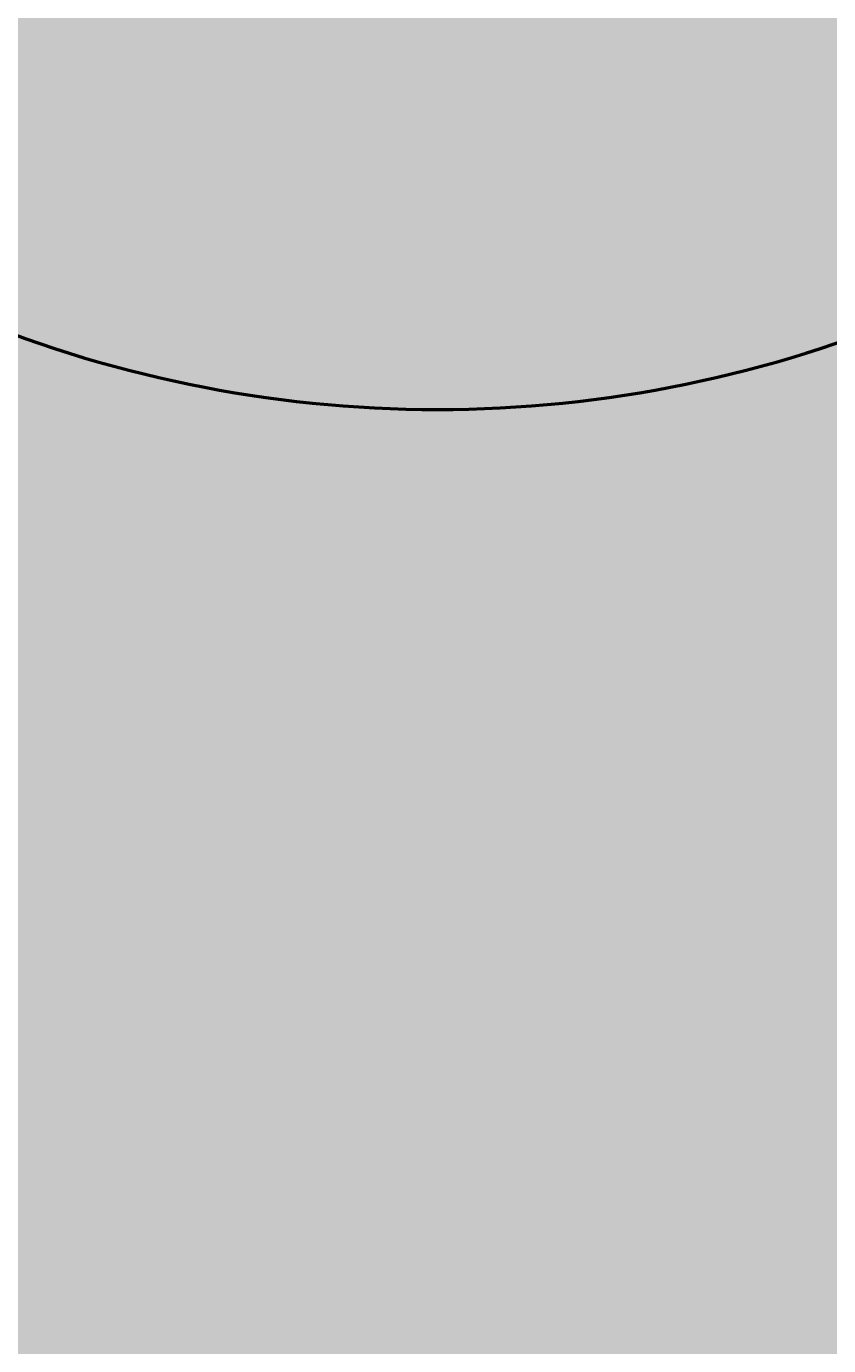
# Model space of a CAD drawing. Units: inches. Extents: x -31 to 87, y -18 to 100.
# Tile 5 of 7: x 18 to 37, y 52 to 84. Entities that reach past the tile are written whole.
import ezdxf

# ---------------------------------------------------------------- set-up
doc = ezdxf.new("R2010")
doc.units = ezdxf.units.IN
doc.header["$MEASUREMENT"] = 0
for name, color, linetype, lineweight in [('M-DIMS', 2, 'Continuous', 18), ('M-HATC', 7, 'Continuous', 18), ('M-OUTL', 4, 'Continuous', 50)]:
    doc.layers.add(name, color=color, linetype=linetype, lineweight=lineweight)
doc.styles.get("Standard").update_dxf_attribs({"font": 'arial.ttf'})
doc.dimstyles.get("Standard").update_dxf_attribs({"dimtxt": 0.18, "dimasz": 0.18, "dimexe": 0.18, "dimexo": 0.0625, "dimgap": 0.09, "dimtad": 0, "dimtih": 1, "dimtoh": 1, "dimdec": 4, "dimzin": 0, "dimdsep": 46, "dimtxsty": 'Standard', "dimcen": 0.09, "dimadec": 0, "dimazin": 0, "dimtfac": 1, "dimtdec": 4, "dimtofl": 0, "dimtmove": 0, "dimatfit": 3, "dimfxl": 1, "dimtolj": 1, "dimtzin": 0, "dimarcsym": 0})

# ---------------------------------------------------------------- blocks, each defined once
blk = doc.blocks.new('*D1')
at = {"layer": 'Defpoints', "color": 0, "transparency": 16777216}
for p in [(-24.622, 75.027), (80.28, 72.235), (80.28, -17.851)]:
    blk.add_point(p, dxfattribs=at)
at = {"layer": 'M-DIMS', "color": 0, "lineweight": -2, "transparency": 16777216}
for p, q in [((-24.622, 74.965), (-24.622, -18.031)), ((80.28, 72.173), (80.28, -18.031)), ((-24.442, -17.851), (27.443, -17.851)), ((80.1, -17.851), (28.214, -17.851))]:
    blk.add_line(p, q, dxfattribs=at)
at = {"layer": 'M-DIMS', "color": 0, "transparency": 16777216}
for points in [[(-24.442, -17.821), (-24.442, -17.881), (-24.622, -17.851)], [(80.1, -17.821), (80.1, -17.881), (80.28, -17.851)]]:
    blk.add_solid(points, dxfattribs=at)
at = {"layer": 'M-DIMS', "color": 0, "transparency": 16777216, "insert": (27.829, -17.851), "char_height": 0.18, "attachment_point": 5}
blk.add_mtext('\\A1;104.9', dxfattribs=at)
blk = doc.blocks.new('*D2')
at = {"layer": 'Defpoints', "color": 0, "transparency": 16777216}
for p in [(60.278, 93.49), (86.68, 93.49), (28.858, -11.451)]:
    blk.add_point(p, dxfattribs=at)
at = {"layer": 'M-DIMS', "color": 0, "lineweight": -2, "transparency": 16777216}
for p, q in [((60.341, 93.49), (86.86, 93.49)), ((86.68, 93.31), (86.68, 41.201)), ((86.68, -11.271), (86.68, 40.838)), ((28.92, -11.451), (86.86, -11.451))]:
    blk.add_line(p, q, dxfattribs=at)
at = {"layer": 'M-DIMS', "color": 0, "transparency": 16777216}
for points in [[(86.65, 93.31), (86.71, 93.31), (86.68, 93.49)], [(86.65, -11.271), (86.71, -11.271), (86.68, -11.451)]]:
    blk.add_solid(points, dxfattribs=at)
at = {"layer": 'M-DIMS', "color": 0, "transparency": 16777216, "insert": (86.68, 41.019), "char_height": 0.18, "attachment_point": 5}
blk.add_mtext('\\A1;104.94', dxfattribs=at)
blk = doc.blocks.new('*D3')
at = {"layer": 'Defpoints', "color": 0, "transparency": 16777216}
for p in [(60.319, 99.89), (-4.681, 73.49), (60.319, 73.49)]:
    blk.add_point(p, dxfattribs=at)
at = {"layer": 'M-DIMS', "color": 0, "lineweight": -2, "transparency": 16777216}
for p, q in [((-4.681, 73.552), (-4.681, 100.07)), ((-4.501, 99.89), (27.599, 99.89)), ((60.139, 99.89), (28.039, 99.89)), ((60.319, 73.552), (60.319, 100.07))]:
    blk.add_line(p, q, dxfattribs=at)
at = {"layer": 'M-DIMS', "color": 0, "transparency": 16777216}
for points in [[(-4.501, 99.92), (-4.501, 99.86), (-4.681, 99.89)], [(60.139, 99.92), (60.139, 99.86), (60.319, 99.89)]]:
    blk.add_solid(points, dxfattribs=at)
at = {"layer": 'M-DIMS', "color": 0, "transparency": 16777216, "insert": (27.819, 99.89), "char_height": 0.18, "attachment_point": 5}
blk.add_mtext('\\A1;65', dxfattribs=at)
blk = doc.blocks.new('*D4')
at = {"layer": 'Defpoints', "color": 0, "transparency": 16777216}
for p in [(-4.681, 73.49), (27.319, 8.49), (27.319, -17.851)]:
    blk.add_point(p, dxfattribs=at)
at = {"layer": 'M-DIMS', "color": 0, "lineweight": -2, "transparency": 16777216}
for p, q in [((-4.681, 73.427), (-4.681, -18.031)), ((27.319, 8.427), (27.319, -18.031)), ((-4.501, -17.851), (11.101, -17.851)), ((27.139, -17.851), (11.537, -17.851))]:
    blk.add_line(p, q, dxfattribs=at)
at = {"layer": 'M-DIMS', "color": 0, "transparency": 16777216}
for points in [[(-4.501, -17.821), (-4.501, -17.881), (-4.681, -17.851)], [(27.139, -17.821), (27.139, -17.881), (27.319, -17.851)]]:
    blk.add_solid(points, dxfattribs=at)
at = {"layer": 'M-DIMS', "color": 0, "transparency": 16777216, "insert": (11.319, -17.851), "char_height": 0.18, "attachment_point": 5}
blk.add_mtext('\\A1;32', dxfattribs=at)
blk = doc.blocks.new('*D5')
at = {"layer": 'Defpoints', "color": 0, "transparency": 16777216}
for p in [(-31.022, 73.49), (-4.681, 73.49), (27.319, 8.49)]:
    blk.add_point(p, dxfattribs=at)
at = {"layer": 'M-DIMS', "color": 0, "lineweight": -2, "transparency": 16777216}
for p, q in [((-4.744, 73.49), (-31.202, 73.49)), ((-31.022, 73.31), (-31.022, 41.172)), ((-31.022, 8.67), (-31.022, 40.808)), ((27.256, 8.49), (-31.202, 8.49))]:
    blk.add_line(p, q, dxfattribs=at)
at = {"layer": 'M-DIMS', "color": 0, "transparency": 16777216}
for points in [[(-31.052, 73.31), (-30.992, 73.31), (-31.022, 73.49)], [(-31.052, 8.67), (-30.992, 8.67), (-31.022, 8.49)]]:
    blk.add_solid(points, dxfattribs=at)
at = {"layer": 'M-DIMS', "color": 0, "transparency": 16777216, "insert": (-31.022, 40.99), "char_height": 0.18, "attachment_point": 5}
blk.add_mtext('\\A1;65', dxfattribs=at)

msp = doc.modelspace()

# ---------------------------------------------------------------- hatches: boundary and pattern name
at = {"layer": 'M-HATC'}
h = msp.add_hatch(color=256, dxfattribs=at)
h.set_gradient(color1=(205, 32, 39), color2=(247, 242, 129))
h.paths.add_polyline_path([(-2.425, 93.362, 0.593504), (-22.614, 64.635), (8.64, 1.342, 0.746388), (46.874, 4.293), (79.436, 67.614, 0.505151), (60.278, 93.49)])
h.paths.add_polyline_path([(49.486, 83.865, -1.392259), (62.663, 58.674, 0.510547), (40.663, 15.341, -1.641082), (14.002, 15.393, 0.505248), (-7.332, 58.726, -1.377138), (6.152, 83.865, 0.426931)], flags=16)
h.paths.add_polyline_path([(5.319, 73.49, -1), (-14.681, 73.49, -1)], flags=0)
h.paths.add_polyline_path([(70.319, 73.49, -1), (50.319, 73.49, -1)], flags=0)
h.paths.add_polyline_path([(37.319, 8.49, -1), (17.319, 8.49, -1)], flags=0)
h.paths.add_polyline_path([(6.152, 83.865, 1.377138), (-7.332, 58.726, -0.505248), (14.002, 15.393, 1.641082), (40.663, 15.341, -0.510547), (62.663, 58.674, 1.392259), (49.486, 83.865, -0.426931)], flags=0)

# ---------------------------------------------------------------- linework, layer by layer
at = {"layer": 'M-OUTL'}
msp.add_arc((27.819, 104.615), 30, 223.7617, 316.2383, dxfattribs=at)

# ---------------------------------------------------------------- dimensions: what is measured, and where the dimension line sits
at = {"layer": 'M-DIMS'}
for base, p1, p2, override, picture, middle in [((60.319, 99.89), (-4.681, 73.49), (60.319, 73.49), {"dimdec": 0, "dimlfac": 1, "dimrnd": 0, "dimzin": 0, "dimdsep": 46, "dimlunit": 2}, '*D3', (27.819, 99.89)), ((80.28, -17.851), (-24.622, 75.027), (80.28, 72.235), {"dimdec": 1, "dimlfac": 1, "dimrnd": 0, "dimzin": 0, "dimdsep": 46, "dimlunit": 2}, '*D1', (27.829, -17.851)), ((27.319, -17.851), (-4.681, 73.49), (27.319, 8.49), {"dimdec": 0, "dimlfac": 1, "dimrnd": 0, "dimzin": 0, "dimdsep": 46, "dimlunit": 2}, '*D4', (11.319, -17.851))]:
    dim = msp.add_linear_dim(base=base, p1=p1, p2=p2, dimstyle='Standard', override=override, dxfattribs=at)
    dim.commit()
    dim.dimension.update_dxf_attribs({"geometry": picture, "text_midpoint": middle})
for base, p1, p2, override, picture, middle in [((86.68, 93.49), (28.858, -11.451), (60.278, 93.49), {"dimdec": 2, "dimlfac": 1, "dimrnd": 0, "dimzin": 0, "dimdsep": 46, "dimlunit": 2}, '*D2', (86.68, 41.019)), ((-31.022, 73.49), (27.319, 8.49), (-4.681, 73.49), {"dimdec": 0, "dimlfac": 1, "dimrnd": 0, "dimzin": 0, "dimdsep": 46, "dimlunit": 2}, '*D5', (-31.022, 40.99))]:
    dim = msp.add_linear_dim(base=base, p1=p1, p2=p2, angle=90, dimstyle='Standard', override=override, dxfattribs=at)
    dim.commit()
    dim.dimension.update_dxf_attribs({"geometry": picture, "text_midpoint": middle})

doc.saveas('drawing.dxf')
